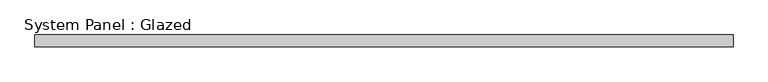
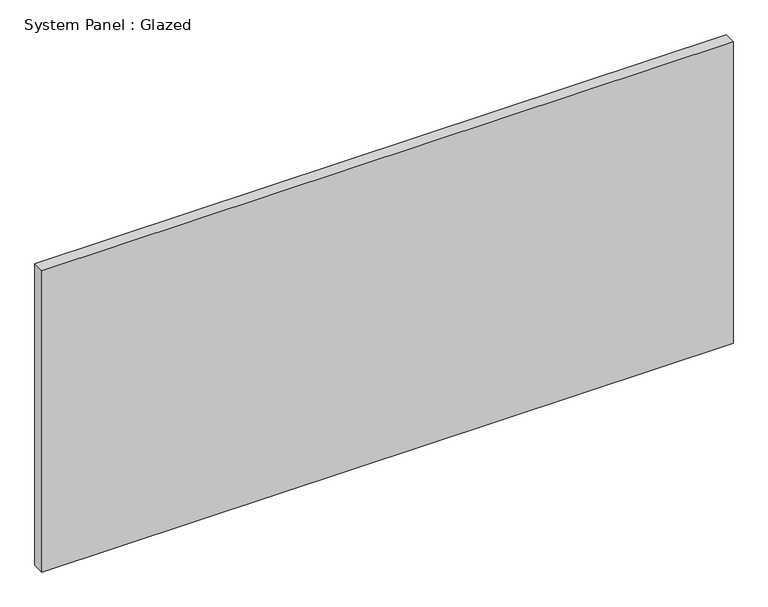
"""IFC4 building model written with IfcOpenShell, lengths in millimetres: plate geometry, System Panel : Glazed."""

from ifc_helpers import new_model, si_unit, origin, origin_with_axes, place, context, project, spatial, polyline, outline, extrude, source, transform, mapped, element, save


def system_panel_glazed_038bf5f5(model_context):
    return source(origin(), model_context, "Body", "SweptSolid", [
        extrude(outline(polyline([(742.95, 19.05), (-742.95, 19.05), (-742.95, 44.45), (742.95, 44.45), (742.95, 19.05)])), origin_with_axes(), (0.0, 0.0, 1.0), 684.9785678),
    ])


if __name__ == "__main__":
    model = new_model("IFC4")
    model_context = context("Model", 3, world=origin())
    ifc_project = project(units=[si_unit("LENGTHUNIT", "METRE", prefix="MILLI")], contexts=[model_context])
    site = spatial("IfcSite", under=ifc_project)
    building = spatial("IfcBuilding", under=site)
    placement = place(None, origin())
    system_panel_glazed_shape = system_panel_glazed_038bf5f5(model_context)
    element("IfcPlate", 1, ObjectType="System Panel : Glazed", at=placement, inside=building, context=model_context, shape_type="MappedRepresentation", body=[
        mapped(system_panel_glazed_shape, transform((0.0, 0.0, 0.0), x_axis=(1.0, 0.0, 0.0), y_axis=(0.0, 1.0, 0.0), z_axis=(0.0, 0.0, 1.0))),
    ])
    save(model, "model.ifc")

# Revit data of these elements
# Type "System Panel : Glazed"
#   Construction Type Id = "GSP4R"
#   Analytic Construction = "1/8 in Pilkington single glazing"
#   Visual Light Transmittance = 0.9
#   Solar Heat Gain Coefficient = 0.86
#   Heat Transfer Coefficient (U) = 1.18115 BTU/(h·ft²·°F)
#   Define Thermal Properties by = 1
# Element 1 (IfcPlate, "System Panel : Glazed")
#   Materials on its faces: "Glass"
# Materials
#   "Glass": class "Glass", colour RGB 0 128 192, transparency 0.75, Description = "Soda Lime Glass", Cost = 0
